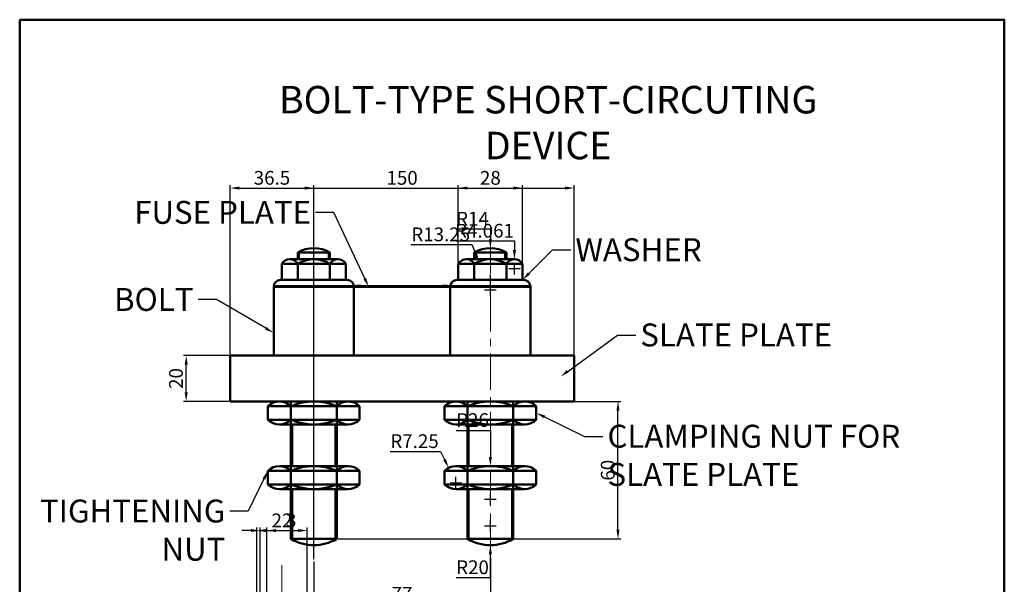
# Model space of a CAD drawing. Units: millimetres. Extents: x 297 to 727, y 87 to 537.
# Tile 2 of 2: x 297 to 727, y 291 to 537. Entities that reach past the tile are written whole.
import ezdxf
from ezdxf import colors
from ezdxf.entities.mleader import LeaderData, LeaderLine
from ezdxf.math import Vec2, Vec3

# ---------------------------------------------------------------- set-up
doc = ezdxf.new("R2010")
doc.units = ezdxf.units.MM
doc.header["$LTSCALE"] = 0.5
doc.linetypes.add('CENTER', pattern=[50.8, 31.75, -6.35, 6.35, -6.35])
for name, color, linetype, lineweight in [('M-CNTR', 1, 'CENTER', 18), ('M-DIMS', 2, 'Continuous', 25), ('M-OUTL', 7, 'Continuous', 50), ('M-TEXT', 3, 'Continuous', 25), ('M-TTLB', 7, 'Continuous', 50)]:
    doc.layers.add(name, color=color, linetype=linetype, lineweight=lineweight)
doc.styles.get("Standard").update_dxf_attribs({"font": 'arial.ttf'})
doc.dimstyles.new('ISO-25', dxfattribs={"dimtxt": 6, "dimasz": 4, "dimexe": 1.25, "dimexo": 0.625, "dimtad": 1, "dimtoh": 1, "dimtxsty": 'Standard', "dimcen": 2.5, "dimadec": 0, "dimazin": 0, "dimtfac": 1, "dimtofl": 0, "dimtmove": 0, "dimatfit": 3, "dimfxl": 1, "dimarcsym": 0})

# ---------------------------------------------------------------- blocks, each defined once
blk = doc.blocks.new('NUT-HEX-M20')
for p, q in [((30, 2), (30, 10)), ((0, 2), (0, 8)), ((0, 8), (40, 8)), ((10, 2), (10, 8)), ((40, 8), (40, 2)), ((40, 2), (0, 2))]:
    blk.add_line(p, q)
for centre, radius, start, end in [((5, 2.75), 7.25, 46.3972, 133.6028), ((20, -16), 26, 67.3801, 112.6199), ((35, 2.75), 7.25, 46.3972, 133.6028), ((5, 7.25), 7.25, 226.3972, 313.6028), ((20, 26), 26, 247.3801, 292.6199), ((35, 7.25), 7.25, 226.3972, 313.6028)]:
    blk.add_arc(centre, radius, start, end)
blk = doc.blocks.new('NUT-HEX-TOP')
for p, q in [((0, 2), (0, 8)), ((0, 8), (40, 8)), ((40, 8), (40, 2)), ((40, 2), (0, 2))]:
    blk.add_line(p, q)
for centre, radius, start, end in [((5, 2.75), 7.25, 46.3972, 133.6028), ((20, -16), 26, 67.3801, 112.6199), ((35, 2.75), 7.25, 46.3972, 133.6028), ((5, 7.25), 7.25, 226.3972, 313.6028), ((20, 26), 26, 247.3801, 292.6199), ((35, 7.25), 7.25, 226.3972, 313.6028)]:
    blk.add_arc(centre, radius, start, end)
blk = doc.blocks.new('BOLT-HEAD-CAP')
for p, q in [((0, 0), (0, 7)), ((0, 7), (28, 7)), ((7, 7), (7, 0)), ((21, 7), (21, 0)), ((28, 0), (28, 7))]:
    blk.add_line(p, q)
for centre, radius, start, end in [((3.5, 4.94), 4.06, 30.4727, 149.5273), ((14, -4.25), 13.25, 58.1092, 121.8908), ((24.5, 4.94), 4.06, 30.4727, 149.5273)]:
    blk.add_arc(centre, radius, start, end)
blk = doc.blocks.new('BOLT-END-DOME')
for p, q in [((0, 3), (0, 0)), ((0, 3), (14, 3)), ((14, 3), (14, 0))]:
    blk.add_line(p, q)
blk.add_arc((7, -9.12), 14, 60, 120)
blk = doc.blocks.new('*D22')
at = {"layer": 'Defpoints', "color": 0, "ltscale": 0.5, "transparency": 16777216}
for p in [(425.71, 463.96), (389.21, 390.88), (425.71, 301.75)]:
    blk.add_point(p, dxfattribs=at)
at = {"layer": 'M-DIMS', "color": 0, "lineweight": -2, "ltscale": 0.5, "transparency": 16777216}
for p, q in [((389.21, 391.5), (389.21, 465.21)), ((393.21, 463.96), (421.71, 463.96)), ((425.71, 302.37), (425.71, 465.21))]:
    blk.add_line(p, q, dxfattribs=at)
at = {"layer": 'M-DIMS', "color": 0, "ltscale": 0.5, "transparency": 16777216}
for points in [[(393.21, 464.62), (393.21, 463.29), (389.21, 463.96)], [(421.71, 464.62), (421.71, 463.29), (425.71, 463.96)]]:
    blk.add_solid(points, dxfattribs=at)
at = {"layer": 'M-DIMS', "color": 0, "ltscale": 0.5, "transparency": 16777216, "insert": (407.46, 467.65), "char_height": 6, "attachment_point": 5}
blk.add_mtext('36.5', dxfattribs=at)
blk = doc.blocks.new('*D23')
at = {"layer": 'Defpoints', "color": 0, "ltscale": 0.5, "transparency": 16777216}
for p in [(425.71, 301.75), (502.71, 303.24), (502.71, 282.6)]:
    blk.add_point(p, dxfattribs=at)
at = {"layer": 'M-DIMS', "color": 0, "lineweight": -2, "ltscale": 0.5, "transparency": 16777216}
for p, q in [((425.71, 301.12), (425.71, 281.35)), ((502.71, 302.61), (502.71, 281.35)), ((429.71, 282.6), (498.71, 282.6))]:
    blk.add_line(p, q, dxfattribs=at)
at = {"layer": 'M-DIMS', "color": 0, "ltscale": 0.5, "transparency": 16777216}
for points in [[(429.71, 283.27), (429.71, 281.93), (425.71, 282.6)], [(498.71, 283.27), (498.71, 281.93), (502.71, 282.6)]]:
    blk.add_solid(points, dxfattribs=at)
at = {"layer": 'M-DIMS', "color": 0, "ltscale": 0.5, "transparency": 16777216, "insert": (464.21, 286.22), "char_height": 6, "attachment_point": 5}
blk.add_mtext('77', dxfattribs=at)
blk = doc.blocks.new('*D24')
at = {"layer": 'Defpoints', "color": 0, "ltscale": 0.5, "transparency": 16777216}
for p in [(539.21, 463.96), (389.21, 370.88), (539.21, 370.88)]:
    blk.add_point(p, dxfattribs=at)
at = {"layer": 'M-DIMS', "color": 0, "lineweight": -2, "ltscale": 0.5, "transparency": 16777216}
for p, q in [((389.21, 371.5), (389.21, 465.21)), ((393.21, 463.96), (535.21, 463.96)), ((539.21, 371.5), (539.21, 465.21))]:
    blk.add_line(p, q, dxfattribs=at)
at = {"layer": 'M-DIMS', "color": 0, "ltscale": 0.5, "transparency": 16777216}
for points in [[(393.21, 464.62), (393.21, 463.29), (389.21, 463.96)], [(535.21, 464.62), (535.21, 463.29), (539.21, 463.96)]]:
    blk.add_solid(points, dxfattribs=at)
at = {"layer": 'M-DIMS', "color": 0, "ltscale": 0.5, "transparency": 16777216, "insert": (464.21, 467.64), "char_height": 6, "attachment_point": 5}
blk.add_mtext('150', dxfattribs=at)
blk = doc.blocks.new('*D25')
at = {"layer": 'Defpoints', "color": 0, "ltscale": 0.5, "transparency": 16777216}
for p in [(440.71, 370.88), (558.36, 370.88), (435.71, 310.88)]:
    blk.add_point(p, dxfattribs=at)
at = {"layer": 'M-DIMS', "color": 0, "lineweight": -2, "ltscale": 0.5, "transparency": 16777216}
for p, q in [((441.33, 370.88), (559.61, 370.88)), ((558.36, 314.88), (558.36, 366.88)), ((436.33, 310.88), (559.61, 310.88))]:
    blk.add_line(p, q, dxfattribs=at)
at = {"layer": 'M-DIMS', "color": 0, "ltscale": 0.5, "transparency": 16777216}
for points in [[(557.69, 366.88), (559.02, 366.88), (558.36, 370.88)], [(557.69, 314.88), (559.02, 314.88), (558.36, 310.88)]]:
    blk.add_solid(points, dxfattribs=at)
at = {"layer": 'M-DIMS', "color": 0, "ltscale": 0.5, "transparency": 16777216, "insert": (554.67, 340.88), "char_height": 6, "attachment_point": 5, "rotation": 90}
blk.add_mtext('60', dxfattribs=at)
blk = doc.blocks.new('*D26')
at = {"layer": 'Defpoints', "color": 0, "ltscale": 0.5, "transparency": 16777216}
for p in [(370.06, 390.88), (389.21, 390.88), (389.21, 370.88)]:
    blk.add_point(p, dxfattribs=at)
at = {"layer": 'M-DIMS', "color": 0, "lineweight": -2, "ltscale": 0.5, "transparency": 16777216}
for p, q in [((388.58, 390.88), (368.81, 390.88)), ((370.06, 374.88), (370.06, 386.88)), ((388.58, 370.88), (368.81, 370.88))]:
    blk.add_line(p, q, dxfattribs=at)
at = {"layer": 'M-DIMS', "color": 0, "ltscale": 0.5, "transparency": 16777216}
for points in [[(369.39, 386.88), (370.72, 386.88), (370.06, 390.88)], [(369.39, 374.88), (370.72, 374.88), (370.06, 370.88)]]:
    blk.add_solid(points, dxfattribs=at)
at = {"layer": 'M-DIMS', "color": 0, "ltscale": 0.5, "transparency": 16777216, "insert": (366.37, 380.88), "char_height": 6, "attachment_point": 5, "rotation": 90}
blk.add_mtext('20', dxfattribs=at)
blk = doc.blocks.new('*D27')
at = {"layer": 'Defpoints', "color": 0, "ltscale": 0.5, "transparency": 16777216}
for p in [(516.71, 463.96), (488.71, 430.88), (516.71, 430.88)]:
    blk.add_point(p, dxfattribs=at)
at = {"layer": 'M-DIMS', "color": 0, "lineweight": -2, "ltscale": 0.5, "transparency": 16777216}
for p, q in [((488.71, 431.5), (488.71, 465.21)), ((492.71, 463.96), (512.71, 463.96)), ((516.71, 431.5), (516.71, 465.21))]:
    blk.add_line(p, q, dxfattribs=at)
at = {"layer": 'M-DIMS', "color": 0, "ltscale": 0.5, "transparency": 16777216}
for points in [[(492.71, 464.62), (492.71, 463.29), (488.71, 463.96)], [(512.71, 464.62), (512.71, 463.29), (516.71, 463.96)]]:
    blk.add_solid(points, dxfattribs=at)
at = {"layer": 'M-DIMS', "color": 0, "ltscale": 0.5, "transparency": 16777216, "insert": (502.71, 467.64), "char_height": 6, "attachment_point": 5}
blk.add_mtext('28', dxfattribs=at)
blk = doc.blocks.new('*D28')
at = {"layer": 'Defpoints', "color": 0, "ltscale": 0.5, "transparency": 16777216}
for p in [(422.82, 314.56), (400.82, 244.11), (422.82, 244.11)]:
    blk.add_point(p, dxfattribs=at)
at = {"layer": 'M-DIMS', "color": 0, "lineweight": -2, "ltscale": 0.5, "transparency": 16777216}
for p, q in [((400.82, 244.73), (400.82, 315.81)), ((404.82, 314.56), (418.82, 314.56)), ((422.82, 244.73), (422.82, 315.81))]:
    blk.add_line(p, q, dxfattribs=at)
at = {"layer": 'M-DIMS', "color": 0, "ltscale": 0.5, "transparency": 16777216}
for points in [[(404.82, 315.23), (404.82, 313.89), (400.82, 314.56)], [(418.82, 315.23), (418.82, 313.89), (422.82, 314.56)]]:
    blk.add_solid(points, dxfattribs=at)
at = {"layer": 'M-DIMS', "color": 0, "ltscale": 0.5, "transparency": 16777216, "insert": (411.82, 318.2), "char_height": 6, "attachment_point": 5}
blk.add_mtext('22', dxfattribs=at)
blk = doc.blocks.new('*D35')
at = {"layer": 'Defpoints', "color": 0, "ltscale": 0.5, "transparency": 16777216}
for p in [(405.26, 314.56), (402.26, 237.29), (405.26, 237.29)]:
    blk.add_point(p, dxfattribs=at)
at = {"layer": 'M-DIMS', "color": 0, "lineweight": -2, "ltscale": 0.5, "transparency": 16777216}
for p, q in [((398.26, 314.56), (394.26, 314.56)), ((402.26, 237.92), (402.26, 315.81)), ((405.26, 237.92), (405.26, 315.81)), ((409.26, 314.56), (418.44, 314.56))]:
    blk.add_line(p, q, dxfattribs=at)
at = {"layer": 'M-DIMS', "color": 0, "ltscale": 0.5, "transparency": 16777216}
for points in [[(398.26, 315.23), (398.26, 313.89), (402.26, 314.56)], [(409.26, 315.23), (409.26, 313.89), (405.26, 314.56)]]:
    blk.add_solid(points, dxfattribs=at)
at = {"layer": 'M-DIMS', "color": 0, "ltscale": 0.5, "transparency": 16777216, "insert": (415.85, 318.25), "char_height": 6, "attachment_point": 5}
blk.add_mtext('3', dxfattribs=at)
blk = doc.blocks.new('*D37')
at = {"layer": 'Defpoints', "color": 0, "ltscale": 0.5, "transparency": 16777216}
for p in [(502.7, 342.67), (502.71, 316.67)]:
    blk.add_point(p, dxfattribs=at)
at = {"layer": 'M-DIMS', "color": 0, "lineweight": -2, "ltscale": 0.5, "transparency": 16777216}
for p, q in [((487.75, 358.27), (502.7, 358.27)), ((502.7, 358.27), (502.7, 346.67)), ((502.71, 314.17), (502.71, 319.17)), ((500.21, 316.67), (505.21, 316.67))]:
    blk.add_line(p, q, dxfattribs=at)
at = {"layer": 'M-DIMS', "color": 0, "ltscale": 0.5, "transparency": 16777216}
blk.add_solid([(503.37, 346.67), (502.04, 346.67), (502.7, 342.67)], dxfattribs=at)
at = {"layer": 'M-DIMS', "color": 0, "ltscale": 0.5, "transparency": 16777216, "insert": (494.91, 361.96), "char_height": 6, "attachment_point": 5}
blk.add_mtext('R26', dxfattribs=at)
blk = doc.blocks.new('*D38')
at = {"layer": 'Defpoints', "color": 0, "ltscale": 0.5, "transparency": 16777216}
for p in [(484.49, 341.92), (487.71, 335.42)]:
    blk.add_point(p, dxfattribs=at)
at = {"layer": 'M-DIMS', "color": 0, "lineweight": -2, "ltscale": 0.5, "transparency": 16777216}
for p, q in [((458.94, 349.09), (480.94, 349.09)), ((480.94, 349.09), (482.72, 345.51)), ((485.21, 335.42), (490.21, 335.42)), ((487.71, 332.92), (487.71, 337.92))]:
    blk.add_line(p, q, dxfattribs=at)
at = {"layer": 'M-DIMS', "color": 0, "ltscale": 0.5, "transparency": 16777216}
blk.add_solid([(483.31, 345.8), (482.12, 345.21), (484.49, 341.92)], dxfattribs=at)
at = {"layer": 'M-DIMS', "color": 0, "ltscale": 0.5, "transparency": 16777216, "insert": (469.63, 352.78), "char_height": 6, "attachment_point": 5}
blk.add_mtext('R7.25', dxfattribs=at)
blk = doc.blocks.new('*D39')
at = {"layer": 'Defpoints', "color": 0, "ltscale": 0.5, "transparency": 16777216}
for p in [(502.71, 328.2), (502.7, 308.2)]:
    blk.add_point(p, dxfattribs=at)
at = {"layer": 'M-DIMS', "color": 0, "lineweight": -2, "ltscale": 0.5, "transparency": 16777216}
for p, q in [((502.71, 325.7), (502.71, 330.7)), ((500.21, 328.2), (505.21, 328.2)), ((502.7, 294.07), (502.7, 304.2)), ((487.76, 294.07), (502.7, 294.07))]:
    blk.add_line(p, q, dxfattribs=at)
at = {"layer": 'M-DIMS', "color": 0, "ltscale": 0.5, "transparency": 16777216}
blk.add_solid([(502.04, 304.2), (503.37, 304.2), (502.7, 308.2)], dxfattribs=at)
at = {"layer": 'M-DIMS', "color": 0, "ltscale": 0.5, "transparency": 16777216, "insert": (494.92, 297.76), "char_height": 6, "attachment_point": 5}
blk.add_mtext('R20', dxfattribs=at)
blk = doc.blocks.new('*D40')
at = {"layer": 'Defpoints', "color": 0, "ltscale": 0.5, "transparency": 16777216}
for p in [(502.7, 437.75), (502.71, 423.75)]:
    blk.add_point(p, dxfattribs=at)
at = {"layer": 'M-DIMS', "color": 0, "lineweight": -2, "ltscale": 0.5, "transparency": 16777216}
for p, q in [((487.77, 446.15), (502.7, 446.15)), ((502.7, 446.15), (502.7, 441.75)), ((502.71, 421.25), (502.71, 426.25)), ((500.21, 423.75), (505.21, 423.75))]:
    blk.add_line(p, q, dxfattribs=at)
at = {"layer": 'M-DIMS', "color": 0, "ltscale": 0.5, "transparency": 16777216}
blk.add_solid([(503.37, 441.75), (502.04, 441.75), (502.7, 437.75)], dxfattribs=at)
at = {"layer": 'M-DIMS', "color": 0, "ltscale": 0.5, "transparency": 16777216, "insert": (494.92, 449.79), "char_height": 6, "attachment_point": 5}
blk.add_mtext('R14', dxfattribs=at)
blk = doc.blocks.new('*D41')
at = {"layer": 'Defpoints', "color": 0, "ltscale": 0.5, "transparency": 16777216}
for p in [(497.71, 431.9), (502.71, 419.63)]:
    blk.add_point(p, dxfattribs=at)
at = {"layer": 'M-DIMS', "color": 0, "lineweight": -2, "ltscale": 0.5, "transparency": 16777216}
for p, q in [((468.03, 439.31), (494.69, 439.31)), ((494.69, 439.31), (496.2, 435.6)), ((502.71, 417.13), (502.71, 422.13)), ((500.21, 419.63), (505.21, 419.63))]:
    blk.add_line(p, q, dxfattribs=at)
at = {"layer": 'M-DIMS', "color": 0, "ltscale": 0.5, "transparency": 16777216}
blk.add_solid([(496.81, 435.85), (495.58, 435.35), (497.71, 431.9)], dxfattribs=at)
at = {"layer": 'M-DIMS', "color": 0, "ltscale": 0.5, "transparency": 16777216, "insert": (481.05, 443), "char_height": 6, "attachment_point": 5}
blk.add_mtext('R13.25', dxfattribs=at)
blk = doc.blocks.new('*D42')
at = {"layer": 'Defpoints', "color": 0, "ltscale": 0.5, "transparency": 16777216}
for p in [(513.2, 432.88), (513.21, 428.82)]:
    blk.add_point(p, dxfattribs=at)
at = {"layer": 'M-DIMS', "color": 0, "lineweight": -2, "ltscale": 0.5, "transparency": 16777216}
for p, q in [((487.75, 440.88), (513.2, 440.88)), ((513.2, 440.88), (513.2, 436.88)), ((513.21, 426.32), (513.21, 431.32)), ((510.71, 428.82), (515.71, 428.82))]:
    blk.add_line(p, q, dxfattribs=at)
at = {"layer": 'M-DIMS', "color": 0, "ltscale": 0.5, "transparency": 16777216}
blk.add_solid([(513.87, 436.88), (512.54, 436.88), (513.2, 432.88)], dxfattribs=at)
at = {"layer": 'M-DIMS', "color": 0, "ltscale": 0.5, "transparency": 16777216, "insert": (500.16, 444.57), "char_height": 6, "attachment_point": 5}
blk.add_mtext('R4.061', dxfattribs=at)

msp = doc.modelspace()

# ---------------------------------------------------------------- linework, layer by layer
at = {"layer": 'M-CNTR'}
for p, q in [((425.7052, 444.8053), (425.7052, 301.7487)), ((502.7052, 442.6055), (502.7052, 303.2378)), ((411.8162, 299.409), (411.8162, 105.0214))]:
    msp.add_line(p, q, dxfattribs=at)
at = {"layer": 'M-OUTL'}
for p, q in [((419.2052, 435.8764), (419.2052, 432.8764)), ((432.2052, 435.8764), (432.2052, 432.8764)), ((496.2052, 435.8764), (496.2052, 432.8764)), ((509.2052, 435.8764), (509.2052, 432.8764)), ((415.0941, 432.8764), (436.3163, 432.8764)), ((492.0941, 432.8764), (513.3163, 432.8764)), ((408.2052, 390.8764), (408.2052, 420.8764)), ((408.2052, 420.8764), (443.2052, 420.8764)), ((411.2052, 423.8764), (440.2052, 423.8764)), ((443.2052, 420.8764), (443.2052, 390.8764)), ((443.2052, 420.8764), (485.2052, 420.8764)), ((485.2052, 390.8764), (485.2052, 420.8764)), ((485.2052, 420.8764), (520.2052, 420.8764)), ((488.2052, 423.8764), (517.2052, 423.8764)), ((520.2052, 420.8764), (520.2052, 390.8764)), ((389.2052, 390.8764), (539.2052, 390.8764)), ((389.2052, 390.8764), (389.2052, 370.8764)), ((424.2052, 390.8764), (389.2052, 390.8764)), ((539.2052, 390.8764), (504.2052, 390.8764)), ((539.2052, 390.8764), (539.2052, 370.8764)), ((539.2052, 370.8764), (389.2052, 370.8764)), ((416.7052, 370.8764), (396.7052, 370.8764)), ((410.7052, 370.8764), (440.7052, 370.8764)), ((415.7052, 370.8764), (415.7052, 310.8764)), ((435.7052, 370.8764), (435.7052, 310.8764)), ((487.7052, 370.8764), (517.7052, 370.8764)), ((492.7052, 370.8764), (492.7052, 310.8764)), ((512.7052, 370.8764), (492.7052, 370.8764)), ((512.7052, 370.8764), (512.7052, 310.8764)), ((435.7052, 358.5799), (435.7052, 366.5799)), ((512.7052, 358.5799), (512.7052, 366.5799)), ((440.7052, 360.8764), (410.7052, 360.8764)), ((415.7052, 358.5799), (415.7052, 364.5799)), ((416.2052, 342.672), (416.2052, 360.8764)), ((435.2052, 360.8764), (435.2052, 342.672)), ((517.7052, 360.8764), (487.7052, 360.8764)), ((492.7052, 358.5799), (492.7052, 364.5799)), ((493.2052, 342.672), (493.2052, 360.8764)), ((512.2052, 360.8764), (512.2052, 342.672)), ((410.7052, 342.672), (440.7052, 342.672)), ((487.7052, 342.672), (517.7052, 342.672)), ((440.7052, 332.672), (410.7052, 332.672)), ((416.2052, 332.672), (416.2052, 310.8764)), ((435.2052, 332.672), (435.2052, 310.8764)), ((517.7052, 332.672), (487.7052, 332.672)), ((493.2052, 332.672), (493.2052, 310.8764)), ((512.2052, 332.672), (512.2052, 310.8764)), ((435.7052, 310.8764), (415.7052, 310.8764)), ((512.7052, 310.8764), (492.7052, 310.8764))]:
    msp.add_line(p, q, dxfattribs=at)
at = {"layer": 'M-OUTL', "ltscale": 0.5}
for p, q in [((482.0323, 421.1264), (408.2156, 421.1264)), ((444.5364, 420.8764), (444.5364, 421.3764)), ((444.5364, 421.3764), (446.3781, 421.3764)), ((446.3781, 421.3764), (446.3781, 420.8764)), ((446.3781, 420.9541), (482.0323, 420.9541)), ((483.874, 421.3764), (482.0323, 421.3764)), ((482.0323, 421.3764), (482.0323, 420.8764)), ((482.0323, 421.1264), (520.2052, 421.1264)), ((483.874, 420.8764), (483.874, 421.3764))]:
    msp.add_line(p, q, dxfattribs=at)
at = {"layer": 'M-OUTL'}
for centre, radius, start, end in [((411.2052, 420.8764), 3, 90, 180), ((440.2052, 420.8764), 3, 0, 90), ((488.2052, 420.8764), 3, 90, 180), ((517.2052, 420.8764), 3, 0, 90), ((425.7052, 328.1969), 20, 240, 300), ((502.7052, 328.1969), 20, 240, 300)]:
    msp.add_arc(centre, radius, start, end, dxfattribs=at)
at = {"layer": 'M-TTLB', "ltscale": 0.5}
msp.add_lwpolyline([(297.4476, 537.4188), (726.8242, 537.4188), (726.8242, 87.0773), (297.4476, 87.0773)], close=True, dxfattribs=at)

# ---------------------------------------------------------------- block references
at = {"layer": 'M-OUTL'}
for name, p in [('BOLT-END-DOME', (418.7048, 432.8764)), ('BOLT-END-DOME', (495.7048, 432.8764)), ('BOLT-HEAD-CAP', (411.705, 423.876)), ('BOLT-HEAD-CAP', (488.705, 423.876)), ('NUT-HEX-TOP', (405.705, 360.876)), ('NUT-HEX-TOP', (482.705, 360.876)), ('NUT-HEX-M20', (405.7048, 332.6715)), ('NUT-HEX-M20', (482.7048, 332.6715))]:
    msp.add_blockref(name, p, dxfattribs=at)

# ---------------------------------------------------------------- texts
at = {"layer": 'M-TEXT', "ltscale": 0.5, "insert": (400.5537, 508.5196), "char_height": 12, "attachment_point": 1}
msp.add_mtext_dynamic_manual_height_columns('\\pxqc;BOLT-TYPE SHORT-CIRCUTING DEVICE', width=254.711718, gutter_width=12.5, heights=[0], dxfattribs=at)

# ---------------------------------------------------------------- dimensions: what is measured, and where the dimension line sits
at = {"layer": 'M-DIMS', "ltscale": 0.5}
for base, p1, p2, override, picture, middle in [((425.7052, 463.9553), (389.2052, 390.8764), (425.7052, 301.7487), {"dimdec": 1, "dimlfac": 1, "dimrnd": 0, "dimzin": 0, "dimdsep": 46, "dimlunit": 2}, '*D22', (407.4552, 467.6458)), ((539.2052, 463.9553), (389.2052, 370.8764), (539.2052, 370.8764), {"dimdec": 0, "dimlfac": 1, "dimrnd": 0, "dimzin": 0, "dimdsep": 46, "dimlunit": 2}, '*D24', (464.2052, 467.6437)), ((516.7052, 463.9553), (488.7052, 430.8764), (516.7052, 430.8764), {"dimdec": 0, "dimlfac": 1, "dimrnd": 0, "dimzin": 0, "dimdsep": 46, "dimlunit": 2}, '*D27', (502.7052, 467.6437)), ((405.2617, 314.559), (402.2617, 237.2918), (405.2617, 237.2918), {"dimdec": 0, "dimlfac": 1, "dimrnd": 0, "dimzin": 0, "dimdsep": 46, "dimlunit": 2}, '*D35', (415.8513, 318.2495)), ((422.8162, 314.559), (400.8162, 244.1085), (422.8162, 244.1085), {"dimdec": 0, "dimlfac": 1, "dimrnd": 0, "dimzin": 0, "dimdsep": 46, "dimlunit": 2}, '*D28', (411.8162, 318.1963)), ((502.7052, 282.5987), (425.7052, 301.7487), (502.7052, 303.2378), {"dimdec": 0, "dimlfac": 1, "dimrnd": 0, "dimzin": 0, "dimdsep": 46, "dimlunit": 2}, '*D23', (464.2052, 286.2237))]:
    dim = msp.add_linear_dim(base=base, p1=p1, p2=p2, dimstyle='ISO-25', override=override, dxfattribs=at)
    dim.commit()
    dim.dimension.update_dxf_attribs({"geometry": picture, "text_midpoint": middle})
for center, mpoint, picture, middle in [((502.7052, 423.752), (502.705, 437.752), '*D40', (494.9237, 446.152)), ((502.7052, 316.672), (502.705, 342.672), '*D37', (494.9134, 358.272))]:
    dim = msp.add_radius_dim(center=center, mpoint=mpoint, dimstyle='ISO-25', override={"dimdec": 0, "dimlfac": 1, "dimrnd": 0, "dimzin": 0, "dimdsep": 46, "dimlunit": 2}, dxfattribs=at)
    dim.commit()
    dim.dimension.update_dxf_attribs({"geometry": picture, "text_midpoint": middle, "dimtype": 164})
for center, mpoint, override, picture, middle in [((502.7052, 419.6264), (497.7062, 431.8972), {"dimdec": 2, "dimlfac": 1, "dimrnd": 0, "dimzin": 0, "dimdsep": 46, "dimlunit": 2}, '*D41', (481.0458, 442.9964)), ((513.2052, 428.817), (513.205, 432.8779), {"dimdec": 3, "dimlfac": 1, "dimrnd": 0, "dimzin": 0, "dimdsep": 46, "dimlunit": 2}, '*D42', (500.1642, 444.5663)), ((487.7052, 335.422), (484.4901, 341.9201), {"dimdec": 2, "dimlfac": 1, "dimrnd": 0, "dimzin": 0, "dimdsep": 46, "dimlunit": 2}, '*D38', (469.6311, 352.7788)), ((502.7052, 328.1969), (502.705, 308.1969), {"dimdec": 0, "dimlfac": 1, "dimrnd": 0, "dimzin": 0, "dimdsep": 46, "dimlunit": 2}, '*D39', (494.9216, 297.7585))]:
    dim = msp.add_radius_dim(center=center, mpoint=mpoint, dimstyle='ISO-25', override=override, dxfattribs=at)
    dim.commit()
    dim.dimension.update_dxf_attribs({"geometry": picture, "text_midpoint": middle})
for base, p1, p2, picture, middle in [((370.0552, 390.8764), (389.2052, 370.8764), (389.2052, 390.8764), '*D26', (366.3668, 380.8764)), ((558.3552, 370.8764), (435.7052, 310.8764), (440.7052, 370.8764), '*D25', (554.6668, 340.8764))]:
    dim = msp.add_linear_dim(base=base, p1=p1, p2=p2, angle=90, dimstyle='ISO-25', override={"dimdec": 0, "dimlfac": 1, "dimrnd": 0, "dimzin": 0, "dimdsep": 46, "dimlunit": 2}, dxfattribs=at)
    dim.commit()
    dim.dimension.update_dxf_attribs({"geometry": picture, "text_midpoint": middle})

# ---------------------------------------------------------------- leaders
at = {"layer": 'M-TEXT', "ltscale": 0.5}
ml = msp.add_multileader_mtext('Standard', dxfattribs=at)
ml.set_content('FUSE PLATE', color=256)
ml.set_leader_properties()
ml.build(insert=Vec2(0, 0))
ctx = ml.context
ctx.base_point, ctx.char_height, ctx.plane_origin = Vec3(339.0053, 453.285), 10, Vec3(449.6287, 420.8764)
ctx.text_align_type = 2
notes = []
notes.append((ctx, [(0, (1, 1, 0), (434.5046, 453.285), (-1, 0), 8, [(0, [(449.6287, 420.8764)], 0, [])])]))
ctx.mtext.insert, ctx.mtext.alignment, ctx.mtext.flow_direction = Vec3(424.5046, 458.3703), 3, 5
ml = msp.add_multileader_mtext('Standard', dxfattribs=at)
ml.set_content('WASHER', color=256)
ml.set_leader_properties()
ml.build(insert=Vec2(0, 0))
ctx = ml.context
ctx.base_point, ctx.char_height, ctx.plane_origin = Vec3(537.8133, 436.9845), 10, Vec3(516.7052, 423.8764)
notes.append((ctx, [(0, (1, 1, 0), (529.8133, 436.9845), (1, 0), 8, [(0, [(516.7052, 423.8764)], 0, [])])]))
ctx.mtext.insert, ctx.mtext.flow_direction = Vec3(539.8133, 442.0697), 5
ml = msp.add_multileader_mtext('Standard', dxfattribs=at)
ml.set_content('BOLT', color=256)
ml.set_leader_properties()
ml.build(insert=Vec2(0, 0))
ctx = ml.context
ctx.base_point, ctx.char_height, ctx.plane_origin = Vec3(336.0589, 415.2909), 10, Vec3(408.2052, 400.7778)
ctx.text_align_type = 2
notes.append((ctx, [(0, (1, 1, 0), (383.243, 415.2909), (-1, 0), 8, [(0, [(408.2052, 400.7778)], 0, [])])]))
ctx.mtext.insert, ctx.mtext.alignment, ctx.mtext.flow_direction = Vec3(373.243, 420.3762), 3, 5
ml = msp.add_multileader_mtext('Standard', dxfattribs=at)
ml.set_content('SLATE PLATE', color=256)
ml.set_leader_properties()
ml.build(insert=Vec2(0, 0))
ctx = ml.context
ctx.base_point, ctx.char_height, ctx.plane_origin = Vec3(566.0716, 399.801), 10, Vec3(533.2003, 381.6425)
notes.append((ctx, [(0, (1, 1, 0), (558.0716, 399.801), (1, 0), 8, [(0, [(533.2003, 381.6425)], 0, [])])]))
ctx.mtext.insert, ctx.mtext.flow_direction = Vec3(568.0716, 404.8862), 5
ml = msp.add_multileader_mtext('Standard', dxfattribs=at)
ml.set_content('CLAMPING NUT FOR \\PSLATE PLATE', color=256)
ml.set_leader_properties()
ml.build(insert=Vec2(0, 0))
ctx = ml.context
ctx.base_point, ctx.char_height, ctx.plane_origin = Vec3(551.7646, 355.6198), 10, Vec3(522.7052, 365.8764)
notes.append((ctx, [(0, (1, 1, 0), (543.7646, 355.6198), (1, 0), 8, [(0, [(522.7052, 365.8764)], 0, [])])]))
ctx.mtext.insert, ctx.mtext.flow_direction = Vec3(553.7646, 360.7051), 5
ml = msp.add_multileader_mtext('Standard', dxfattribs=at)
ml.set_content('TIGHTENING \\PNUT', color=256)
ml.set_leader_properties()
ml.build(insert=Vec2(0, 0))
ctx = ml.context
ctx.base_point, ctx.char_height, ctx.plane_origin = Vec3(300.202, 322.9915), 10, Vec3(332.6652, 336.2987)
ctx.text_align_type = 2
notes.append((ctx, [(1, (1, 1, 0), (397.1475, 322.9915), (-1, 0), 8, [(0, [(405.7052, 340.672)], 0, [])])]))
ctx.mtext.insert, ctx.mtext.alignment, ctx.mtext.flow_direction = Vec3(387.1475, 328.0768), 3, 5
for ctx, leaders in notes:
    for number, flags, end, landing, length, lines in leaders:
        leader = LeaderData()
        leader.index, (leader.has_last_leader_line, leader.has_dogleg_vector, leader.attachment_direction) = number, flags
        leader.last_leader_point, leader.dogleg_vector, leader.dogleg_length = Vec3(end), Vec3(landing), length
        for number, points, colour, breaks in lines:
            line = LeaderLine()
            line.index, line.vertices, line.color, line.breaks = number, Vec3.list(points), colors.encode_raw_color(colour), breaks
            leader.lines.append(line)
        ctx.leaders.append(leader)

doc.saveas('drawing.dxf')
